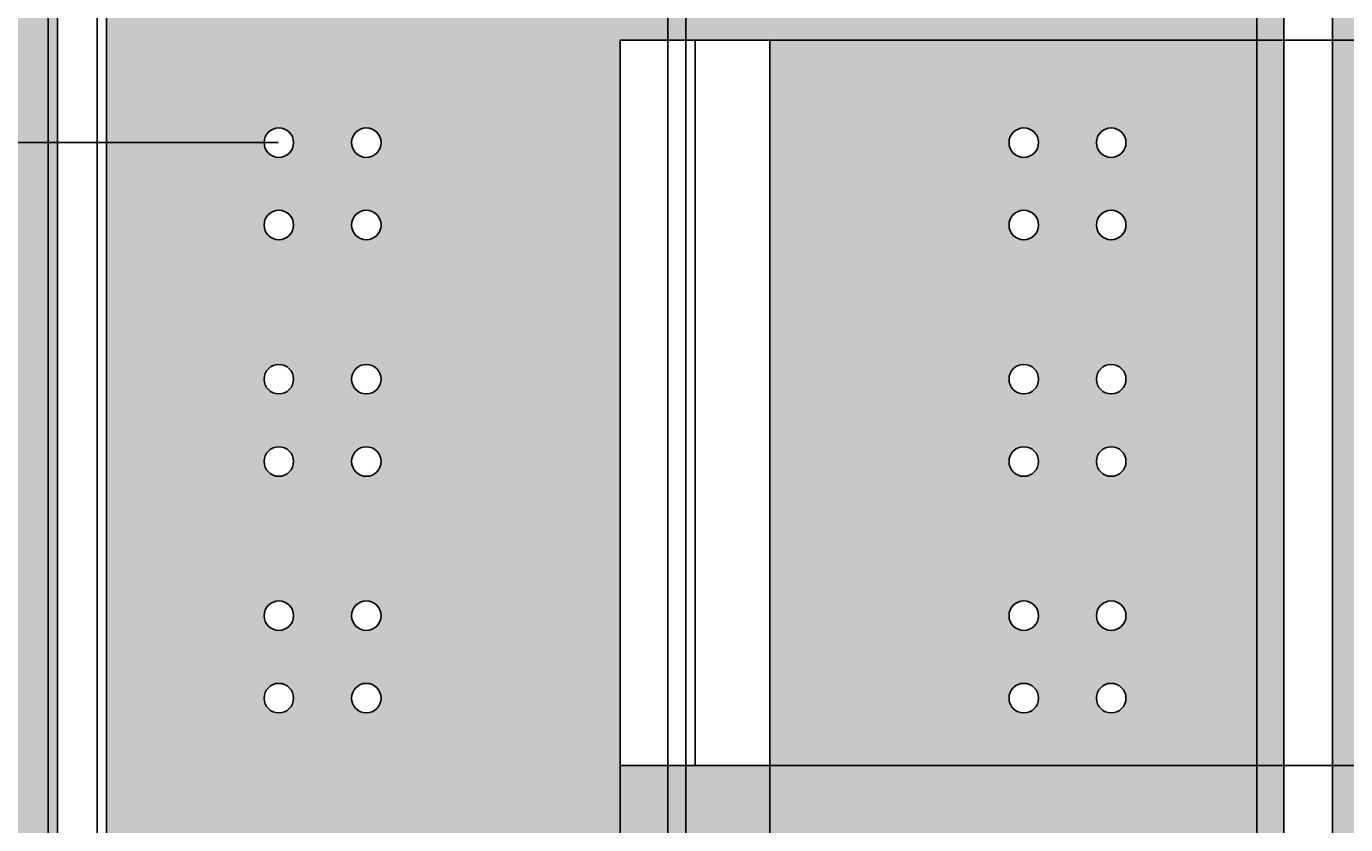
# Model space of a CAD drawing. Units: inches. Extents: x 3024 to 4744, y 1110 to 2100.
# Tile 5 of 29: x 3168 to 3275, y 1181 to 1246. Entities that reach past the tile are written whole.
import ezdxf

# ---------------------------------------------------------------- set-up
doc = ezdxf.new("R2010")
doc.units = ezdxf.units.IN
for name, color, linetype, lineweight in [('A-ANNO-DIMS', 2, 'Continuous', 18), ('A-ELEV', 7, 'Continuous', 25), ('A-ELEV-PATT', 252, 'Continuous', 13)]:
    doc.layers.add(name, color=color, linetype=linetype, lineweight=lineweight)
doc.styles.get("Standard").update_dxf_attribs({"font": 'arial.ttf'})
doc.dimstyles.get("Standard").update_dxf_attribs({"dimtxt": 0.18, "dimasz": 0.18, "dimexe": 0.18, "dimexo": 0.0625, "dimgap": 0.09, "dimtad": 0, "dimtih": 1, "dimtoh": 1, "dimdec": 1, "dimzin": 0, "dimdsep": 46, "dimlunit": 3, "dimtxsty": 'Standard', "dimcen": 0.09, "dimadec": 0, "dimazin": 0, "dimtfac": 1, "dimtdec": 1, "dimtofl": 0, "dimtmove": 0, "dimatfit": 3, "dimfxl": 1, "dimtolj": 1, "dimtzin": 0, "dimarcsym": 0})

# ---------------------------------------------------------------- blocks, each defined once
blk = doc.blocks.new('*D52')
at = {"layer": 'A-ANNO-DIMS', "color": 0, "lineweight": -2, "transparency": 16777216}
for p, q in [((3148.97, 1290.98), (3148.97, 1109.93)), ((3170.16, 1170.96), (3170.16, 1109.93)), ((3149.15, 1110.11), (3159.17, 1110.11)), ((3169.98, 1110.11), (3159.96, 1110.11))]:
    blk.add_line(p, q, dxfattribs=at)
at = {"layer": 'A-ANNO-DIMS', "color": 0, "transparency": 16777216}
for points in [[(3149.15, 1110.14), (3149.15, 1110.08), (3148.97, 1110.11)], [(3169.98, 1110.14), (3169.98, 1110.08), (3170.16, 1110.11)]]:
    blk.add_solid(points, dxfattribs=at)
at = {"layer": 'Defpoints', "color": 0, "transparency": 16777216}
for p in [(3148.97, 1291.04), (3170.16, 1171.02), (3170.16, 1110.11)]:
    blk.add_point(p, dxfattribs=at)
at = {"layer": 'A-ANNO-DIMS', "color": 0, "transparency": 16777216, "insert": (3159.57, 1110.11), "char_height": 0.18, "attachment_point": 5}
blk.add_mtext('\\A1;21.19', dxfattribs=at)
blk = doc.blocks.new('*D54')
at = {"layer": 'A-ANNO-DIMS', "color": 0, "lineweight": -2, "transparency": 16777216}
for p, q in [((3292.61, 1290.98), (3292.61, 1109.93)), ((3274.39, 1170.96), (3274.39, 1109.93)), ((3274.57, 1110.11), (3283.04, 1110.11)), ((3292.43, 1110.11), (3283.95, 1110.11))]:
    blk.add_line(p, q, dxfattribs=at)
at = {"layer": 'A-ANNO-DIMS', "color": 0, "transparency": 16777216}
for points in [[(3274.57, 1110.14), (3274.57, 1110.08), (3274.39, 1110.11)], [(3292.43, 1110.14), (3292.43, 1110.08), (3292.61, 1110.11)]]:
    blk.add_solid(points, dxfattribs=at)
at = {"layer": 'Defpoints', "color": 0, "transparency": 16777216}
for p in [(3292.61, 1291.04), (3274.39, 1171.02), (3292.61, 1110.11)]:
    blk.add_point(p, dxfattribs=at)
at = {"layer": 'A-ANNO-DIMS', "color": 0, "transparency": 16777216, "insert": (3283.5, 1110.11), "char_height": 0.18, "attachment_point": 5}
blk.add_mtext('\\A1;18.217', dxfattribs=at)
blk = doc.blocks.new('*D64')
at = {"layer": 'A-ANNO-DIMS', "color": 0, "lineweight": -2, "transparency": 16777216}
for p, q in [((3069.79, 1241.5), (3069.79, 2100.44)), ((3741.15, 1241.5), (3741.15, 2100.44)), ((3069.97, 2100.26), (3405.08, 2100.26)), ((3740.97, 2100.26), (3405.87, 2100.26))]:
    blk.add_line(p, q, dxfattribs=at)
at = {"layer": 'A-ANNO-DIMS', "color": 0, "transparency": 16777216}
for points in [[(3069.97, 2100.29), (3069.97, 2100.23), (3069.79, 2100.26)], [(3740.97, 2100.29), (3740.97, 2100.23), (3741.15, 2100.26)]]:
    blk.add_solid(points, dxfattribs=at)
at = {"layer": 'Defpoints', "color": 0, "transparency": 16777216}
for p in [(3741.15, 2100.26), (3069.79, 1241.43), (3741.15, 1241.43)]:
    blk.add_point(p, dxfattribs=at)
at = {"layer": 'A-ANNO-DIMS', "color": 0, "transparency": 16777216, "insert": (3405.47, 2100.26), "char_height": 0.18, "attachment_point": 5}
blk.add_mtext('\\A1;671.4', dxfattribs=at)
blk = doc.blocks.new('*D90')
at = {"layer": 'A-ANNO-DIMS', "color": 0, "lineweight": -2, "transparency": 16777216}
for p, q in [((3173.4, 1798.98), (3173.4, 1109.93)), ((3169.4, 1794.98), (3169.4, 1109.93)), ((3169.58, 1110.11), (3171.07, 1110.11)), ((3173.22, 1110.11), (3171.72, 1110.11))]:
    blk.add_line(p, q, dxfattribs=at)
at = {"layer": 'A-ANNO-DIMS', "color": 0, "transparency": 16777216}
for points in [[(3169.58, 1110.14), (3169.58, 1110.08), (3169.4, 1110.11)], [(3173.22, 1110.14), (3173.22, 1110.08), (3173.4, 1110.11)]]:
    blk.add_solid(points, dxfattribs=at)
at = {"layer": 'Defpoints', "color": 0, "transparency": 16777216}
for p in [(3173.4, 1799.04), (3169.4, 1795.04), (3173.4, 1110.11)]:
    blk.add_point(p, dxfattribs=at)
at = {"layer": 'A-ANNO-DIMS', "color": 0, "transparency": 16777216, "insert": (3171.4, 1110.11), "char_height": 0.18, "attachment_point": 5}
blk.add_mtext('\\A1;4.00', dxfattribs=at)
blk = doc.blocks.new('*D91')
at = {"layer": 'A-ANNO-DIMS', "color": 0, "lineweight": -2, "transparency": 16777216}
for p, q in [((3173.4, 1798.98), (3173.4, 1109.93)), ((3220.05, 1798.98), (3220.05, 1109.93)), ((3173.58, 1110.11), (3196.33, 1110.11)), ((3219.87, 1110.11), (3197.12, 1110.11))]:
    blk.add_line(p, q, dxfattribs=at)
at = {"layer": 'A-ANNO-DIMS', "color": 0, "transparency": 16777216}
for points in [[(3173.58, 1110.14), (3173.58, 1110.08), (3173.4, 1110.11)], [(3219.87, 1110.14), (3219.87, 1110.08), (3220.05, 1110.11)]]:
    blk.add_solid(points, dxfattribs=at)
at = {"layer": 'Defpoints', "color": 0, "transparency": 16777216}
for p in [(3173.4, 1799.04), (3220.05, 1799.04), (3220.05, 1110.11)]:
    blk.add_point(p, dxfattribs=at)
at = {"layer": 'A-ANNO-DIMS', "color": 0, "transparency": 16777216, "insert": (3196.72, 1110.11), "char_height": 0.18, "attachment_point": 5}
blk.add_mtext('\\A1;46.65', dxfattribs=at)
blk = doc.blocks.new('*D92')
at = {"layer": 'A-ANNO-DIMS', "color": 0, "lineweight": -2, "transparency": 16777216}
for p, q in [((3220.05, 1798.98), (3220.05, 1109.93)), ((3221.52, 1798.98), (3221.52, 1109.93)), ((3220.23, 1110.11), (3220.47, 1110.11)), ((3221.34, 1110.11), (3221.1, 1110.11))]:
    blk.add_line(p, q, dxfattribs=at)
at = {"layer": 'A-ANNO-DIMS', "color": 0, "transparency": 16777216}
for points in [[(3220.23, 1110.14), (3220.23, 1110.08), (3220.05, 1110.11)], [(3221.34, 1110.14), (3221.34, 1110.08), (3221.52, 1110.11)]]:
    blk.add_solid(points, dxfattribs=at)
at = {"layer": 'Defpoints', "color": 0, "transparency": 16777216}
for p in [(3220.05, 1799.04), (3221.52, 1799.04), (3221.52, 1110.11)]:
    blk.add_point(p, dxfattribs=at)
at = {"layer": 'A-ANNO-DIMS', "color": 0, "transparency": 16777216, "insert": (3220.79, 1110.11), "char_height": 0.18, "attachment_point": 5}
blk.add_mtext('\\A1;1.47', dxfattribs=at)
blk = doc.blocks.new('*D93')
at = {"layer": 'A-ANNO-DIMS', "color": 0, "lineweight": -2, "transparency": 16777216}
for p, q in [((3221.52, 1798.98), (3221.52, 1109.93)), ((3268.18, 1798.98), (3268.18, 1109.93)), ((3221.7, 1110.11), (3244.45, 1110.11)), ((3268, 1110.11), (3245.25, 1110.11))]:
    blk.add_line(p, q, dxfattribs=at)
at = {"layer": 'A-ANNO-DIMS', "color": 0, "transparency": 16777216}
for points in [[(3221.7, 1110.14), (3221.7, 1110.08), (3221.52, 1110.11)], [(3268, 1110.14), (3268, 1110.08), (3268.18, 1110.11)]]:
    blk.add_solid(points, dxfattribs=at)
at = {"layer": 'Defpoints', "color": 0, "transparency": 16777216}
for p in [(3221.52, 1799.04), (3268.18, 1799.04), (3268.18, 1110.11)]:
    blk.add_point(p, dxfattribs=at)
at = {"layer": 'A-ANNO-DIMS', "color": 0, "transparency": 16777216, "insert": (3244.85, 1110.11), "char_height": 0.18, "attachment_point": 5}
blk.add_mtext('\\A1;46.65', dxfattribs=at)
blk = doc.blocks.new('*D109')
at = {"layer": 'A-ANNO-DIMS', "color": 0, "lineweight": -2, "transparency": 16777216}
for p, q in [((3216.16, 1185.89), (3216.16, 1109.93)), ((3228.39, 1185.89), (3228.39, 1109.93)), ((3216.34, 1110.11), (3221.82, 1110.11)), ((3228.21, 1110.11), (3222.73, 1110.11))]:
    blk.add_line(p, q, dxfattribs=at)
at = {"layer": 'A-ANNO-DIMS', "color": 0, "transparency": 16777216}
for points in [[(3216.34, 1110.14), (3216.34, 1110.08), (3216.16, 1110.11)], [(3228.21, 1110.14), (3228.21, 1110.08), (3228.39, 1110.11)]]:
    blk.add_solid(points, dxfattribs=at)
at = {"layer": 'Defpoints', "color": 0, "transparency": 16777216}
for p in [(3216.16, 1185.95), (3228.39, 1185.95), (3228.39, 1110.11)]:
    blk.add_point(p, dxfattribs=at)
at = {"layer": 'A-ANNO-DIMS', "color": 0, "transparency": 16777216, "insert": (3222.27, 1110.11), "char_height": 0.18, "attachment_point": 5}
blk.add_mtext('\\A1;12.223', dxfattribs=at)
blk = doc.blocks.new('*D120')
at = {"layer": 'A-ANNO-DIMS', "color": 0, "lineweight": -2, "transparency": 16777216}
for p, q in [((3270.45, 1271.61), (3786.83, 1271.61)), ((3786.65, 1271.43), (3786.65, 1221.5)), ((3786.65, 1171.2), (3786.65, 1221.14)), ((3274.45, 1171.02), (3786.83, 1171.02))]:
    blk.add_line(p, q, dxfattribs=at)
at = {"layer": 'A-ANNO-DIMS', "color": 0, "transparency": 16777216}
for points in [[(3786.62, 1271.43), (3786.68, 1271.43), (3786.65, 1271.61)], [(3786.62, 1171.2), (3786.68, 1171.2), (3786.65, 1171.02)]]:
    blk.add_solid(points, dxfattribs=at)
at = {"layer": 'Defpoints', "color": 0, "transparency": 16777216}
for p in [(3270.39, 1271.61), (3786.65, 1271.61), (3274.39, 1171.02)]:
    blk.add_point(p, dxfattribs=at)
at = {"layer": 'A-ANNO-DIMS', "color": 0, "transparency": 16777216, "insert": (3786.65, 1221.32), "char_height": 0.18, "attachment_point": 5}
blk.add_mtext('\\A1;100.59', dxfattribs=at)
blk = doc.blocks.new('*D122')
at = {"layer": 'A-ANNO-DIMS', "color": 0, "lineweight": -2, "transparency": 16777216}
for p, q in [((3228.45, 1185.95), (3786.83, 1185.95)), ((3786.65, 1185.77), (3786.65, 1178.67)), ((3786.65, 1171.2), (3786.65, 1178.31)), ((3270.45, 1171.02), (3786.83, 1171.02))]:
    blk.add_line(p, q, dxfattribs=at)
at = {"layer": 'A-ANNO-DIMS', "color": 0, "transparency": 16777216}
for points in [[(3786.62, 1185.77), (3786.68, 1185.77), (3786.65, 1185.95)], [(3786.62, 1171.2), (3786.68, 1171.2), (3786.65, 1171.02)]]:
    blk.add_solid(points, dxfattribs=at)
at = {"layer": 'Defpoints', "color": 0, "transparency": 16777216}
for p in [(3228.39, 1185.95), (3270.39, 1171.02), (3786.65, 1171.02)]:
    blk.add_point(p, dxfattribs=at)
at = {"layer": 'A-ANNO-DIMS', "color": 0, "transparency": 16777216, "insert": (3786.65, 1178.49), "char_height": 0.18, "attachment_point": 5}
blk.add_mtext('\\A1;14.928', dxfattribs=at)
blk = doc.blocks.new('*D123')
at = {"layer": 'A-ANNO-DIMS', "color": 0, "lineweight": -2, "transparency": 16777216}
for p, q in [((3228.45, 1245.27), (3786.83, 1245.27)), ((3786.65, 1245.09), (3786.65, 1215.79)), ((3786.65, 1186.13), (3786.65, 1215.43)), ((3228.45, 1185.95), (3786.83, 1185.95))]:
    blk.add_line(p, q, dxfattribs=at)
at = {"layer": 'A-ANNO-DIMS', "color": 0, "transparency": 16777216}
for points in [[(3786.62, 1245.09), (3786.68, 1245.09), (3786.65, 1245.27)], [(3786.62, 1186.13), (3786.68, 1186.13), (3786.65, 1185.95)]]:
    blk.add_solid(points, dxfattribs=at)
at = {"layer": 'Defpoints', "color": 0, "transparency": 16777216}
for p in [(3228.39, 1245.27), (3786.65, 1245.27), (3228.39, 1185.95)]:
    blk.add_point(p, dxfattribs=at)
at = {"layer": 'A-ANNO-DIMS', "color": 0, "transparency": 16777216, "insert": (3786.65, 1215.61), "char_height": 0.18, "attachment_point": 5}
blk.add_mtext('\\A1;59.32', dxfattribs=at)
blk = doc.blocks.new('*D129')
at = {"layer": 'A-ANNO-DIMS', "color": 0, "lineweight": -2, "transparency": 16777216}
for p, q in [((3188.2, 1249.49), (3024.11, 1249.49)), ((3024.29, 1249.31), (3024.29, 1243.37)), ((3024.29, 1237.07), (3024.29, 1243.01)), ((3188.2, 1236.89), (3024.11, 1236.89))]:
    blk.add_line(p, q, dxfattribs=at)
at = {"layer": 'A-ANNO-DIMS', "color": 0, "transparency": 16777216}
for points in [[(3024.26, 1249.31), (3024.32, 1249.31), (3024.29, 1249.49)], [(3024.26, 1237.07), (3024.32, 1237.07), (3024.29, 1236.89)]]:
    blk.add_solid(points, dxfattribs=at)
at = {"layer": 'Defpoints', "color": 0, "transparency": 16777216}
for p in [(3188.26, 1249.49), (3024.29, 1236.89), (3188.26, 1236.89)]:
    blk.add_point(p, dxfattribs=at)
at = {"layer": 'A-ANNO-DIMS', "color": 0, "transparency": 16777216, "insert": (3024.29, 1243.19), "char_height": 0.18, "attachment_point": 5}
blk.add_mtext('\\A1;12.603', dxfattribs=at)

msp = doc.modelspace()

# ---------------------------------------------------------------- hatches: boundary and pattern name
at = {"layer": 'A-ELEV-PATT'}
h = msp.add_hatch(color=256, dxfattribs=at)
h.dxf.hatch_style = 1
h.paths.add_polyline_path([(3329.7033, 1275.6112), (3274.3877, 1275.6112), (3274.3877, 1171.0239), (3329.7033, 1171.0239)])
h.paths.add_polyline_path([(3323.3693, 1246.0161), (3279.3584, 1246.0161), (3279.3584, 1270.5642), (3323.3693, 1270.5642)], flags=16)
h.paths.add_polyline_path([(3323.3693, 1238.118), (3323.3693, 1213.5699), (3279.3584, 1213.5699), (3279.3584, 1238.118)], flags=16)
h.paths.add_polyline_path([(3323.3693, 1205.6718), (3323.3693, 1181.1236), (3279.3584, 1181.1236), (3279.3584, 1205.6718)], flags=16)
h.paths.add_polyline_path([(3170.1608, 1275.6112), (3112.3838, 1275.6112), (3112.3838, 1171.0239), (3118.1176, 1171.0239), (3170.1608, 1171.0239)])
h.paths.add_polyline_path([(3120.3696, 1246.0161), (3120.3696, 1270.5642), (3164.3806, 1270.5642), (3164.3806, 1246.0161)], flags=16)
h.paths.add_polyline_path([(3120.3696, 1238.118), (3164.3806, 1238.118), (3164.3806, 1213.5699), (3120.3696, 1213.5699)], flags=16)
h.paths.add_polyline_path([(3120.3696, 1205.6718), (3164.3806, 1205.6718), (3164.3806, 1181.1236), (3120.3696, 1181.1236)], flags=16)
h = msp.add_hatch(color=256, dxfattribs=at)
h.dxf.hatch_style = 1
h.paths.add_polyline_path([(3270.3877, 1271.6112), (3174.1608, 1271.6112), (3174.1608, 1171.0239), (3187.7692, 1171.0239, -0.29659686), (3187.0515, 1172.1274, -1), (3189.4658, 1172.1274, -0.29659686), (3188.7481, 1171.0239), (3194.9159, 1171.0239, -0.29659686), (3194.1982, 1172.1274, -1), (3196.6124, 1172.1274, -0.29659686), (3195.8947, 1171.0239), (3248.6539, 1171.0239, -0.29659686), (3247.9362, 1172.1274, -1), (3250.3504, 1172.1274, -0.29659686), (3249.6327, 1171.0239), (3255.8005, 1171.0239, -0.29659686), (3255.0828, 1172.1274, -1), (3257.4971, 1172.1274, -0.29659686), (3256.7794, 1171.0239), (3270.3877, 1171.0239)])
h.paths.add_polyline_path([(3196.6124, 1256.2276, -1), (3194.1982, 1256.2276, -1)], flags=16)
h.paths.add_polyline_path([(3196.6124, 1249.4899, -1), (3194.1982, 1249.4899, -1)], flags=16)
h.paths.add_polyline_path([(3216.163, 1245.2708), (3228.3856, 1245.2708), (3228.3856, 1185.9515), (3216.163, 1185.9515)], flags=16)
h.paths.add_polyline_path([(3187.0515, 1256.2276, -1), (3189.4658, 1256.2276, -1)], flags=16)
h.paths.add_polyline_path([(3189.4658, 1249.4899, -1), (3187.0515, 1249.4899, -1)], flags=16)
h.paths.add_polyline_path([(3196.6124, 1236.8869, -1), (3194.1982, 1236.8869, -1)], flags=16)
h.paths.add_polyline_path([(3189.4658, 1236.8869, -1), (3187.0515, 1236.8869, -1)], flags=16)
h.paths.add_polyline_path([(3196.6124, 1230.1493, -1), (3194.1982, 1230.1493, -1)], flags=16)
h.paths.add_polyline_path([(3189.4658, 1230.1493, -1), (3187.0515, 1230.1493, -1)], flags=16)
h.paths.add_polyline_path([(3250.3504, 1256.2276, -1), (3247.9362, 1256.2276, -1)], flags=16)
h.paths.add_polyline_path([(3250.3504, 1249.4899, -1), (3247.9362, 1249.4899, -1)], flags=16)
h.paths.add_polyline_path([(3196.6124, 1217.5463, -1), (3194.1982, 1217.5463, -1)], flags=16)
h.paths.add_polyline_path([(3250.3504, 1236.8869, -1), (3247.9362, 1236.8869, -1)], flags=16)
h.paths.add_polyline_path([(3189.4658, 1217.5463, -1), (3187.0515, 1217.5463, -1)], flags=16)
h.paths.add_polyline_path([(3257.4971, 1256.2276, -1), (3255.0828, 1256.2276, -1)], flags=16)
h.paths.add_polyline_path([(3257.4971, 1249.4899, -1), (3255.0828, 1249.4899, -1)], flags=16)
h.paths.add_polyline_path([(3250.3504, 1230.1493, -1), (3247.9362, 1230.1493, -1)], flags=16)
h.paths.add_polyline_path([(3196.6124, 1210.8086, -1), (3194.1982, 1210.8086, -1)], flags=16)
h.paths.add_polyline_path([(3189.4658, 1210.8086, -1), (3187.0515, 1210.8086, -1)], flags=16)
h.paths.add_polyline_path([(3257.4971, 1236.8869, -1), (3255.0828, 1236.8869, -1)], flags=16)
h.paths.add_polyline_path([(3257.4971, 1230.1493, -1), (3255.0828, 1230.1493, -1)], flags=16)
h.paths.add_polyline_path([(3250.3504, 1217.5463, -1), (3247.9362, 1217.5463, -1)], flags=16)
h.paths.add_polyline_path([(3196.6124, 1198.2057, -1), (3194.1982, 1198.2057, -1)], flags=16)
h.paths.add_polyline_path([(3250.3504, 1210.8086, -1), (3247.9362, 1210.8086, -1)], flags=16)
h.paths.add_polyline_path([(3257.4971, 1217.5463, -1), (3255.0828, 1217.5463, -1)], flags=16)
h.paths.add_polyline_path([(3189.4658, 1198.2057, -1), (3187.0515, 1198.2057, -1)], flags=16)
h.paths.add_polyline_path([(3257.4971, 1210.8086, -1), (3255.0828, 1210.8086, -1)], flags=16)
h.paths.add_polyline_path([(3196.6124, 1191.468, -1), (3194.1982, 1191.468, -1)], flags=16)
h.paths.add_polyline_path([(3189.4658, 1191.468, -1), (3187.0515, 1191.468, -1)], flags=16)
h.paths.add_polyline_path([(3250.3504, 1198.2057, -1), (3247.9362, 1198.2057, -1)], flags=16)
h.paths.add_polyline_path([(3257.4971, 1198.2057, -1), (3255.0828, 1198.2057, -1)], flags=16)
h.paths.add_polyline_path([(3250.3504, 1191.468, -1), (3247.9362, 1191.468, -1)], flags=16)
h.paths.add_polyline_path([(3196.6124, 1178.8651, -1), (3194.1982, 1178.8651, -1)], flags=16)
h.paths.add_polyline_path([(3257.4971, 1191.468, -1), (3255.0828, 1191.468, -1)], flags=16)
h.paths.add_polyline_path([(3189.4658, 1178.8651, -1), (3187.0515, 1178.8651, -1)], flags=16)
h.paths.add_polyline_path([(3250.3504, 1178.8651, -1), (3247.9362, 1178.8651, -1)], flags=16)
h.paths.add_polyline_path([(3257.4971, 1178.8651, -1), (3255.0828, 1178.8651, -1)], flags=16)

# ---------------------------------------------------------------- linework, layer by layer
at = {"layer": 'A-ELEV'}
msp.add_line((3222.2743, 1245.2708), (3222.2743, 1185.9515), dxfattribs=at)
msp.add_line((3222.2743, 1245.2708), (3222.2743, 1185.9515), dxfattribs=at)
for points in [[(3170.1608, 1171.0239), (3170.1608, 1275.6112), (3274.3877, 1275.6112), (3274.3877, 1171.0239)], [(3170.1608, 1171.0239), (3170.1608, 1275.6112), (3274.3877, 1275.6112), (3274.3877, 1171.0239)], [(3174.1608, 1171.0239), (3174.1608, 1271.6112), (3270.3877, 1271.6112), (3270.3877, 1171.0239)], [(3174.1608, 1171.0239), (3174.1608, 1271.6112), (3270.3877, 1271.6112), (3270.3877, 1171.0239)]]:
    msp.add_lwpolyline(points, dxfattribs=at)
msp.add_lwpolyline([(3228.3856, 1185.9515), (3216.163, 1185.9515), (3216.163, 1245.2708), (3228.3856, 1245.2708)], close=True, dxfattribs=at)
msp.add_lwpolyline([(3228.3856, 1185.9515), (3216.163, 1185.9515), (3216.163, 1245.2708), (3228.3856, 1245.2708)], close=True, dxfattribs=at)
for centre in [(3188.2586, 1236.8869), (3188.2586, 1236.8869), (3195.4053, 1236.8869), (3195.4053, 1236.8869), (3249.1433, 1236.8869), (3249.1433, 1236.8869), (3256.2899, 1236.8869), (3256.2899, 1236.8869), (3188.2586, 1230.1493), (3188.2586, 1230.1493), (3195.4053, 1230.1493), (3195.4053, 1230.1493), (3249.1433, 1230.1493), (3249.1433, 1230.1493), (3256.2899, 1230.1493), (3256.2899, 1230.1493), (3188.2586, 1217.5463), (3188.2586, 1217.5463), (3195.4053, 1217.5463), (3195.4053, 1217.5463), (3249.1433, 1217.5463), (3249.1433, 1217.5463), (3256.2899, 1217.5463), (3256.2899, 1217.5463), (3188.2586, 1210.8086), (3188.2586, 1210.8086), (3195.4053, 1210.8086), (3195.4053, 1210.8086), (3249.1433, 1210.8086), (3249.1433, 1210.8086), (3256.2899, 1210.8086), (3256.2899, 1210.8086), (3188.2586, 1198.2057), (3188.2586, 1198.2057), (3195.4053, 1198.2057), (3195.4053, 1198.2057), (3249.1433, 1198.2057), (3249.1433, 1198.2057), (3256.2899, 1198.2057), (3256.2899, 1198.2057), (3188.2586, 1191.468), (3188.2586, 1191.468), (3195.4053, 1191.468), (3195.4053, 1191.468), (3249.1433, 1191.468), (3249.1433, 1191.468), (3256.2899, 1191.468), (3256.2899, 1191.468)]:
    msp.add_circle(centre, 1.2071, dxfattribs=at)

# ---------------------------------------------------------------- dimensions: what is measured, and where the dimension line sits
at = {"layer": 'A-ANNO-DIMS'}
for base, p1, p2, override, picture, middle in [((3741.1507, 2100.2584), (3069.7937, 1241.4341), (3741.1507, 1241.4341), {"dimdec": 1, "dimlfac": 1, "dimrnd": 0, "dimzin": 0, "dimdsep": 46, "dimlunit": 2}, '*D64', (3405.4722, 2100.2584)), ((3173.3964, 1110.1112), (3169.3964, 1795.0431), (3173.3964, 1799.0431), {"dimdec": 2, "dimlfac": 1, "dimrnd": 0, "dimzin": 0, "dimdsep": 46, "dimlunit": 2}, '*D90', (3171.3964, 1110.1112)), ((3220.0505, 1110.1112), (3173.3964, 1799.0431), (3220.0505, 1799.0431), {"dimdec": 2, "dimlfac": 1, "dimrnd": 0, "dimzin": 0, "dimdsep": 46, "dimlunit": 2}, '*D91', (3196.7234, 1110.1112)), ((3221.5241, 1110.1112), (3220.0505, 1799.0431), (3221.5241, 1799.0431), {"dimdec": 2, "dimlfac": 1, "dimrnd": 0, "dimzin": 0, "dimdsep": 46, "dimlunit": 2}, '*D92', (3220.7873, 1110.1112)), ((3268.1781, 1110.1112), (3221.5241, 1799.0431), (3268.1781, 1799.0431), {"dimdec": 2, "dimlfac": 1, "dimrnd": 0, "dimzin": 0, "dimdsep": 46, "dimlunit": 2}, '*D93', (3244.8511, 1110.1112)), ((3170.1608, 1110.1112), (3148.9694, 1291.0431), (3170.1608, 1171.0239), {"dimdec": 2, "dimlfac": 1, "dimrnd": 0, "dimzin": 0, "dimdsep": 46, "dimlunit": 2}, '*D52', (3159.5651, 1110.1112)), ((3292.6051, 1110.1112), (3274.3877, 1171.0239), (3292.6051, 1291.0431), {"dimdec": 3, "dimlfac": 1, "dimrnd": 0, "dimzin": 0, "dimdsep": 46, "dimlunit": 2}, '*D54', (3283.4964, 1110.1112)), ((3228.3856, 1110.1112), (3216.163, 1185.9515), (3228.3856, 1185.9515), {"dimdec": 3, "dimlfac": 1, "dimrnd": 0, "dimzin": 0, "dimdsep": 46, "dimlunit": 2}, '*D109', (3222.2743, 1110.1112))]:
    dim = msp.add_linear_dim(base=base, p1=p1, p2=p2, dimstyle='Standard', override=override, dxfattribs=at)
    dim.commit()
    dim.dimension.update_dxf_attribs({"geometry": picture, "text_midpoint": middle})
for base, p1, p2, override, picture, middle in [((3786.6507, 1271.6112), (3274.3877, 1171.0239), (3270.3877, 1271.6112), {"dimdec": 2, "dimlfac": 1, "dimrnd": 0, "dimzin": 0, "dimdsep": 46, "dimlunit": 2}, '*D120', (3786.6507, 1221.3176)), ((3024.2937, 1236.8869), (3188.2586, 1249.4899), (3188.2586, 1236.8869), {"dimdec": 3, "dimlfac": 1, "dimrnd": 0, "dimzin": 0, "dimdsep": 46, "dimlunit": 2}, '*D129', (3024.2937, 1243.1884)), ((3786.6507, 1245.2708), (3228.3856, 1185.9515), (3228.3856, 1245.2708), {"dimdec": 2, "dimlfac": 1, "dimrnd": 0, "dimzin": 0, "dimdsep": 46, "dimlunit": 2}, '*D123', (3786.6507, 1215.6112)), ((3786.6507, 1171.0239), (3228.3856, 1185.9515), (3270.3877, 1171.0239), {"dimdec": 3, "dimlfac": 1, "dimrnd": 0, "dimzin": 0, "dimdsep": 46, "dimlunit": 2}, '*D122', (3786.6507, 1178.4877))]:
    dim = msp.add_linear_dim(base=base, p1=p1, p2=p2, angle=90, dimstyle='Standard', override=override, dxfattribs=at)
    dim.commit()
    dim.dimension.update_dxf_attribs({"geometry": picture, "text_midpoint": middle})

doc.saveas('drawing.dxf')
